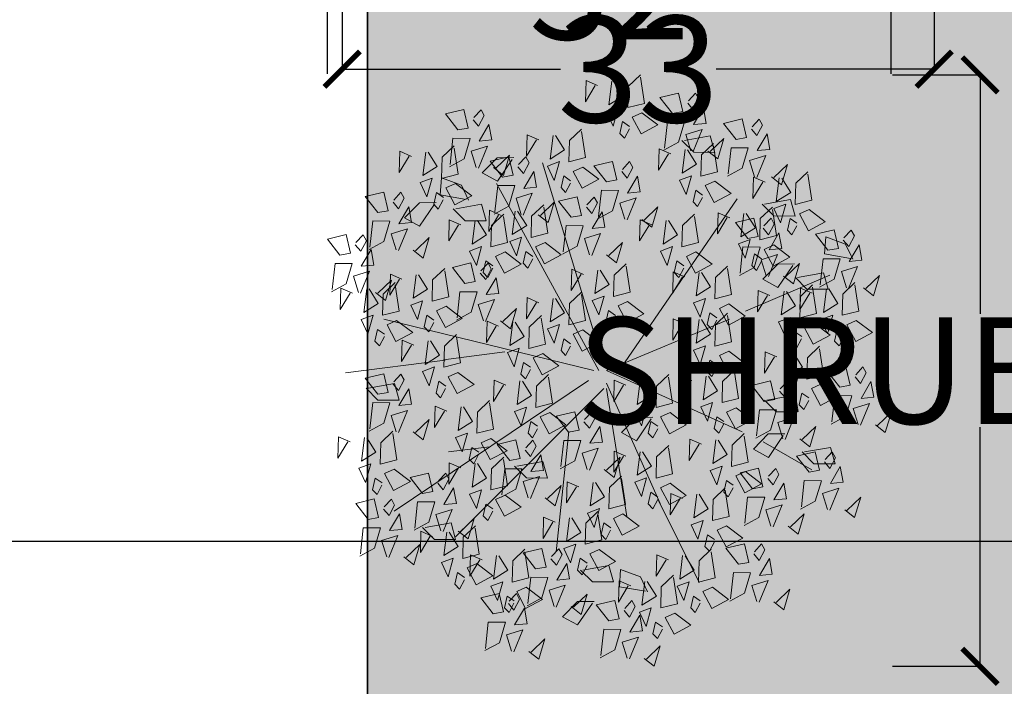
# Model space of a CAD drawing. Units: inches. Extents: x 1704 to 6393, y -157 to 1172.
# Tile 10 of 122: x 1879 to 1934, y 82 to 120. Entities that reach past the tile are written whole.
import ezdxf

# ---------------------------------------------------------------- set-up
doc = ezdxf.new("R2010")
doc.units = ezdxf.units.IN
doc.header["$MEASUREMENT"] = 0
for name, color, linetype, lineweight in [('A-ANNO-DIMS', 7, 'Continuous', 13), ('C-PROP', 7, 'Continuous', 35), ('L-shrub', 74, 'Continuous', 18)]:
    doc.layers.add(name, color=color, linetype=linetype, lineweight=lineweight)
doc.layers.add('L-PLNT-PATT', color=253, linetype='Continuous', lineweight=13, true_color=0x9abc8f)
doc.styles.get("Standard").update_dxf_attribs({"font": 'arial.ttf'})
doc.dimstyles.get("Standard").update_dxf_attribs({"dimtxt": 6, "dimasz": 2, "dimexe": 0.18, "dimexo": 0.0625, "dimgap": 0.09, "dimtad": 0, "dimtih": 1, "dimtoh": 1, "dimdec": 1, "dimzin": 0, "dimdsep": 46, "dimlunit": 3, "dimtxsty": 'Standard', "dimblk": 'ARCHTICK', "dimcen": 0.09, "dimadec": 0, "dimazin": 0, "dimtfac": 1, "dimtdec": 1, "dimtofl": 0, "dimtmove": 0, "dimatfit": 3, "dimfxl": 1, "dimtolj": 1, "dimtzin": 0, "dimarcsym": 0})

# ---------------------------------------------------------------- blocks, each defined once
blk = doc.blocks.new('flower shrub 2')
at = {"layer": 'L-shrub'}
for p, q in [((-106.23, 211.82), (-92.99, 218)), ((-93.69, 216.06), (-97.6, 193.26)), ((-112.6, 194.32), (-106.23, 211.82)), ((71.95, 198.59), (86.43, 202.67)), ((75.99, 175.82), (71.95, 198.59)), ((86.43, 202.67), (86.36, 184.05)), ((-97.6, 193.26), (-112.6, 194.32)), ((-81.12, 192.39), (-66.64, 196.47)), ((-77.07, 169.62), (-81.12, 192.39)), ((-66.64, 196.47), (-66.71, 177.85)), ((86.36, 184.05), (75.99, 173.75)), ((-66.71, 177.85), (-77.08, 167.55)), ((-145.24, 163.47), (-130.76, 167.54)), ((-130.76, 167.54), (-130.83, 148.93)), ((-88.72, 152.29), (-88.87, 166.9)), ((-87.4, 165.46), (-68.26, 152.47)), ((26.45, 165.53), (40.92, 169.61)), ((30.49, 142.76), (26.45, 165.53)), ((40.92, 169.61), (40.85, 150.99)), ((-141.2, 140.7), (-145.24, 163.47)), ((60.21, 144.02), (60.06, 158.64)), ((61.53, 157.19), (80.67, 144.21)), ((-130.83, 148.93), (-141.21, 138.63)), ((-75.44, 139.25), (-88.72, 152.29)), ((-68.26, 152.47), (-75.44, 139.25)), ((40.85, 150.99), (30.48, 140.69)), ((73.5, 130.99), (60.21, 144.02)), ((80.67, 144.21), (73.5, 130.99)), ((-201.09, 93.22), (-186.61, 97.3)), ((-186.61, 97.3), (-186.68, 78.69)), ((-197.05, 70.45), (-201.09, 93.22)), ((-186.68, 78.69), (-197.06, 68.38)), ((45.73, 28.33), (45.58, 42.95)), ((47.06, 41.5), (66.19, 28.51)), ((185.43, 32.08), (198.67, 38.26)), ((197.96, 36.32), (194.06, 13.53)), ((59.02, 15.29), (45.73, 28.33)), ((66.19, 28.51), (59.02, 15.29)), ((179.06, 14.59), (185.43, 32.08)), ((194.06, 13.53), (179.06, 14.59)), ((175.38, 4.39), (189.86, 8.47)), ((179.42, -18.38), (175.38, 4.39)), ((189.86, 8.47), (189.78, -10.15)), ((189.78, -10.15), (179.41, -20.45)), ((207.07, -23.32), (206.92, -8.7)), ((208.4, -10.15), (227.53, -23.13)), ((220.36, -36.35), (207.07, -23.32)), ((227.53, -23.13), (220.36, -36.35)), ((84.36, -53.46), (98.84, -49.38)), ((98.84, -49.38), (98.77, -68)), ((88.41, -76.23), (84.36, -53.46)), ((98.77, -68), (88.4, -78.3)), ((-181.81, -93.56), (-181.96, -78.94)), ((-180.48, -80.39), (-161.34, -93.38)), ((-168.52, -106.6), (-181.81, -93.56)), ((-161.34, -93.38), (-168.52, -106.6)), ((-141.1, -107.17), (-126.62, -103.09)), ((-126.62, -103.09), (-126.7, -121.71)), ((-137.06, -129.94), (-141.1, -107.17)), ((-157.94, -124.93), (-144.7, -118.75)), ((-145.41, -120.69), (-149.31, -143.48)), ((-164.31, -142.42), (-157.94, -124.93)), ((-126.7, -121.71), (-137.07, -132.01)), ((138.15, -134.03), (152.62, -129.95)), ((142.19, -156.8), (138.15, -134.03)), ((152.62, -129.95), (152.55, -148.57)), ((-149.31, -143.48), (-164.31, -142.42)), ((-142.51, -161.74), (-142.65, -147.12)), ((-141.18, -148.57), (-122.04, -161.55)), ((152.55, -148.57), (142.18, -158.87)), ((-129.22, -174.77), (-142.51, -161.74)), ((-122.04, -161.55), (-129.22, -174.77)), ((16.1, -183.61), (30.58, -179.53)), ((30.58, -179.53), (30.51, -198.15)), ((20.14, -206.38), (16.1, -183.61)), ((30.51, -198.15), (20.14, -208.45))]:
    blk.add_line(p, q, dxfattribs=at)
for points in [[(52.15, 237.83), (59.05, 246.56), (41.2, 251.84), (52.74, 239.81)], [(-67.82, 227.5), (-60.92, 236.23), (-78.77, 241.51), (-67.23, 229.48)], [(-39.32, 221.12), (-28.59, 235.29), (-20.71, 220.61), (-35.41, 212.74), (-39.32, 221.12)], [(29.03, 225.28), (27.99, 236.36), (14.33, 233.94), (29.03, 225.28)], [(-90.95, 214.95), (-91.98, 226.03), (-105.64, 223.61), (-90.95, 214.95)], [(10.23, 220.07), (15.95, 224.84), (6.62, 229.76), (1.48, 226.97), (8.24, 220.66)], [(52.02, 222.79), (37.77, 218.39), (33.35, 232.62), (52.6, 224.77)], [(126.62, 210.97), (133.52, 219.7), (115.67, 224.99), (127.2, 212.95)], [(-109.75, 209.74), (-104.02, 214.51), (-113.35, 219.43), (-118.49, 216.64), (-111.73, 210.33)], [(-67.96, 212.46), (-82.2, 208.06), (-86.62, 222.29), (-67.37, 214.44)], [(-70.39, 219.89), (-47.54, 223.41), (-43.79, 208.84), (-62.4, 209.34), (-72.46, 219.95)], [(19.2, 206.65), (5.18, 195.71), (1.34, 211.93), (17.57, 215.74), (19.2, 206.65)], [(49.53, 199.82), (26.54, 202.32), (26.68, 217.36), (44.53, 212.08), (51.52, 199.24)], [(-27.19, 210.46), (-31.5, 204.37), (-21.21, 202.03), (-16.97, 206.05), (-25.13, 210.4)], [(103.49, 198.43), (102.46, 209.5), (88.8, 207.08), (103.49, 198.43)], [(-100.78, 196.32), (-114.8, 185.38), (-118.63, 201.6), (-102.4, 205.41), (-100.78, 196.32)], [(-70.44, 189.49), (-93.43, 191.99), (-93.29, 207.03), (-75.44, 201.75), (-68.45, 188.91)], [(-66.87, 197.06), (-54.24, 204.99), (-46.3, 192.37), (-66.93, 195)], [(-44.01, 200.58), (-40.16, 190.14), (-27.58, 196), (-44.01, 200.58)], [(16.53, 190.13), (27.26, 204.31), (35.14, 189.63), (20.44, 181.76), (16.53, 190.13)], [(84.69, 193.22), (90.42, 197.99), (81.09, 202.9), (75.95, 200.11), (82.71, 193.8)], [(126.48, 195.93), (112.24, 191.53), (107.82, 205.76), (127.07, 197.91)], [(-136.54, 179.8), (-125.81, 193.98), (-117.93, 179.3), (-132.63, 171.43), (-136.54, 179.8)], [(-47.57, 123.92), (-79, 197.93)], [(-37.25, 183.93), (-26.52, 198.11), (-18.64, 183.43), (-33.34, 175.56), (-37.25, 183.93)], [(-14.54, 188.9), (8.31, 192.42), (12.06, 177.85), (-6.55, 178.35), (-16.61, 188.96)], [(124, 172.97), (101.01, 175.46), (101.15, 190.5), (119, 185.22), (125.98, 172.38)], [(-167.61, 178.57), (-144.76, 182.09), (-141.01, 167.52), (-159.62, 168.02), (-169.68, 178.63)], [(-68.32, 182.7), (-45.47, 186.22), (-41.72, 171.65), (-60.33, 172.15), (-70.39, 182.76)], [(-63.13, 182.49), (-67.54, 172.28), (-48.93, 171.78), (-63.18, 180.43)], [(64.56, 171.72), (71.46, 180.45), (53.61, 185.73), (65.15, 173.7)], [(66.94, 139.62), (91.63, 182.23)], [(93.66, 179.79), (79.64, 168.86), (75.81, 185.07), (92.04, 188.89), (93.66, 179.79)], [(-25.12, 173.27), (-29.43, 167.19), (-19.14, 164.84), (-14.9, 168.86), (-23.06, 173.21)], [(-11.02, 166.07), (1.61, 174), (9.54, 161.38), (-11.08, 164.01)], [(28.66, 179.47), (24.35, 173.38), (34.64, 171.04), (38.88, 175.06), (30.72, 179.41)], [(141.1, 161.39), (148, 170.12), (130.14, 175.4), (141.68, 163.37)], [(-124.41, 169.14), (-128.72, 163.05), (-118.43, 160.71), (-114.19, 164.73), (-122.34, 169.08)], [(-78.16, 157.26), (-71.26, 165.99), (-89.12, 171.27), (-77.58, 159.24)], [(-64.8, 159.87), (-52.17, 167.8), (-44.24, 155.19), (-64.86, 157.81)], [(11.84, 169.59), (15.69, 159.15), (28.27, 165.01), (11.84, 169.59)], [(41.44, 159.17), (40.4, 170.25), (26.74, 167.83), (41.44, 159.17)], [(64.43, 156.68), (50.18, 152.28), (45.76, 166.51), (65.01, 158.66)], [(-165.04, 146.93), (-158.14, 155.66), (-175.99, 160.94), (-164.45, 148.91)], [(-164.09, 155.74), (-151.46, 163.67), (-143.52, 151.05), (-164.15, 153.68)], [(-141.23, 159.26), (-137.38, 148.82), (-124.8, 154.68), (-141.23, 159.26)], [(-101.29, 144.71), (-102.33, 155.79), (-115.98, 153.37), (-101.29, 144.71)], [(-105.51, 148.81), (-94.78, 162.99), (-86.9, 148.31), (-101.6, 140.44), (-105.51, 148.81)], [(-41.95, 163.39), (-38.09, 152.95), (-25.52, 158.81), (-41.95, 163.39)], [(22.64, 153.96), (28.36, 158.73), (19.03, 163.65), (13.89, 160.86), (20.65, 154.55)], [(117.97, 148.84), (116.93, 159.92), (103.28, 157.5), (117.97, 148.84)], [(140.96, 146.35), (126.72, 141.95), (122.3, 156.18), (141.55, 148.33)], [(207.29, 148.99), (214.19, 157.72), (196.34, 163.01), (207.88, 150.97)], [(-136.58, 147.58), (-113.73, 151.1), (-109.98, 136.53), (-128.59, 137.03), (-138.65, 147.64)], [(-120.09, 139.5), (-114.36, 144.27), (-123.69, 149.19), (-128.83, 146.4), (-122.07, 140.09)], [(-78.3, 142.22), (-92.54, 137.81), (-96.96, 152.05), (-77.71, 144.2)], [(-7.28, 151.5), (-11.69, 141.29), (6.92, 140.79), (-7.33, 149.44)], [(31.61, 140.54), (17.59, 129.6), (13.76, 145.82), (29.99, 149.63), (31.61, 140.54)], [(61.95, 133.71), (38.95, 136.21), (39.09, 151.25), (56.94, 145.97), (63.93, 133.13)], [(99.17, 143.63), (104.9, 148.4), (95.57, 153.32), (90.43, 150.53), (97.19, 144.22)], [(184.16, 136.45), (183.13, 147.53), (169.47, 145.1), (184.16, 136.45)], [(-206.97, 129.17), (-201.24, 133.94), (-210.57, 138.86), (-215.71, 136.07), (-208.95, 129.76)], [(-188.17, 134.38), (-189.2, 145.46), (-202.86, 143.04), (-188.17, 134.38)], [(-165.18, 131.89), (-179.42, 127.48), (-183.84, 141.72), (-164.59, 133.87)], [(-160.34, 141.17), (-164.76, 130.96), (-146.15, 130.46), (-160.4, 139.11)], [(-93.39, 138.15), (-97.69, 132.06), (-87.4, 129.72), (-83.16, 133.74), (-91.32, 138.09)], [(-61.06, 145.31), (-65.47, 135.09), (-46.86, 134.59), (-61.11, 143.24)], [(108.14, 130.21), (94.12, 119.27), (90.29, 135.49), (106.52, 139.3), (108.14, 130.21)], [(93.06, 124.02), (103.79, 138.2), (111.67, 123.52), (96.98, 115.65), (93.06, 124.02)], [(138.48, 123.38), (115.49, 125.88), (115.63, 140.92), (133.48, 135.64), (140.46, 122.8)], [(165.36, 131.24), (171.09, 136.01), (161.76, 140.92), (156.62, 138.13), (163.38, 131.82)], [(207.15, 133.95), (192.91, 129.55), (188.49, 143.78), (207.74, 135.93)], [(-133.06, 124.75), (-120.43, 132.68), (-112.5, 120.06), (-133.12, 122.69)], [(-111.12, 126.07), (-125.14, 115.14), (-128.97, 131.36), (-112.74, 135.17), (-111.12, 126.07)], [(-80.78, 119.25), (-103.77, 121.75), (-103.63, 136.79), (-85.78, 131.5), (-78.8, 118.66)], [(37.21, 115.75), (47.94, 129.93), (55.82, 115.25), (41.13, 107.38), (37.21, 115.75)], [(-198, 115.75), (-212.02, 104.81), (-215.85, 121.03), (-199.62, 124.84), (-198, 115.75)], [(-167.66, 108.92), (-190.65, 111.42), (-190.51, 126.46), (-172.66, 121.17), (-165.67, 108.33)], [(-110.21, 128.27), (-106.35, 117.83), (-93.78, 123.69), (-110.21, 128.27)], [(-53.8, 109.56), (-43.07, 123.73), (-35.19, 109.05), (-49.89, 101.18), (-53.8, 109.56)], [(-12.43, 109.56), (-1.7, 123.73), (6.18, 109.05), (-8.52, 101.18), (-12.43, 109.56)], [(4.49, 2.24), (58.38, 121.09)], [(61.99, 122.79), (84.85, 126.31), (88.59, 111.74), (69.98, 112.24), (59.92, 122.85)], [(140.64, 107.49), (151.37, 121.67), (159.25, 106.99), (144.55, 99.12), (140.64, 107.49)], [(174.33, 117.81), (160.31, 106.88), (156.48, 123.09), (172.71, 126.91), (174.33, 117.81)], [(204.67, 110.99), (181.68, 113.48), (181.82, 128.52), (199.67, 123.24), (206.65, 110.4)], [(-2.25, 17.94), (-145.94, 116.61)], [(6.14, 114.53), (29, 118.04), (32.74, 103.47), (14.13, 103.98), (4.07, 114.58)], [(105.19, 113.36), (100.89, 107.27), (111.17, 104.93), (115.42, 108.95), (107.26, 113.3)], [(-187.79, 91.15), (-180.89, 99.88), (-198.75, 105.16), (-187.21, 93.13)], [(-161.36, 97.16), (-150.63, 111.34), (-142.75, 96.66), (-157.45, 88.79), (-161.36, 97.16)], [(-129.32, 110.18), (-133.73, 99.97), (-115.12, 99.47), (-129.37, 108.12)], [(-84.87, 108.33), (-62.02, 111.85), (-58.27, 97.28), (-76.88, 97.78), (-86.94, 108.38)], [(-43.5, 108.33), (-20.65, 111.85), (-16.9, 97.28), (-35.51, 97.78), (-45.57, 108.38)], [(4.49, 2.24), (-40.41, 109.88)], [(49.34, 105.09), (45.04, 99.01), (55.32, 96.67), (59.57, 100.68), (51.41, 105.04)], [(65.51, 99.96), (78.14, 107.89), (86.08, 95.27), (65.46, 97.9)], [(109.57, 106.26), (132.42, 109.78), (136.17, 95.21), (117.56, 95.71), (107.5, 106.32)], [(194.42, 95.09), (205.15, 109.27), (213.03, 94.59), (198.33, 86.72), (194.42, 95.09)], [(-192.43, 95.93), (-169.58, 99.45), (-165.83, 84.88), (-184.44, 85.38), (-194.5, 95.99)], [(-41.67, 98.9), (-45.98, 92.81), (-35.69, 90.47), (-31.45, 94.49), (-39.6, 98.84)], [(-0.3, 98.9), (-4.61, 92.81), (5.68, 90.47), (9.92, 94.49), (1.76, 98.84)], [(9.66, 91.7), (22.29, 99.62), (30.23, 87.01), (9.61, 89.63)], [(32.52, 95.21), (36.38, 84.78), (48.95, 90.64), (32.52, 95.21)], [(88.37, 103.48), (92.23, 93.04), (104.8, 98.9), (88.37, 103.48)], [(152.77, 96.83), (148.46, 90.75), (158.75, 88.4), (162.99, 92.42), (154.83, 96.77)], [(163.35, 93.87), (186.2, 97.38), (189.95, 82.82), (171.34, 83.32), (161.28, 93.92)], [(-210.92, 78.6), (-211.96, 89.68), (-225.62, 87.26), (-210.92, 78.6)], [(-149.23, 86.5), (-153.54, 80.42), (-143.25, 78.07), (-139.01, 82.09), (-147.17, 86.44)], [(-99.31, 80.63), (-88.58, 94.81), (-80.7, 80.13), (-95.39, 72.26), (-99.31, 80.63)], [(-81.35, 85.5), (-68.72, 93.43), (-60.78, 80.81), (-81.41, 83.43)], [(-58.49, 89.02), (-54.64, 78.58), (-42.06, 84.44), (-58.49, 89.02)], [(-39.98, 85.5), (-27.35, 93.43), (-19.41, 80.81), (-40.04, 83.43)], [(-17.12, 89.02), (-13.27, 78.58), (-0.69, 84.44), (-17.12, 89.02)], [(113.09, 83.43), (125.72, 91.36), (133.65, 78.75), (113.03, 81.37)], [(135.94, 86.95), (139.8, 76.51), (152.38, 82.37), (135.94, 86.95)], [(-229.72, 73.39), (-223.99, 78.16), (-233.32, 83.08), (-238.46, 80.29), (-231.7, 73.98)], [(-187.93, 76.11), (-202.17, 71.7), (-206.59, 85.94), (-187.34, 78.09)], [(-188.91, 73.1), (-176.28, 81.03), (-168.35, 68.42), (-188.97, 71.04)], [(-130.38, 79.41), (-107.52, 82.92), (-103.78, 68.35), (-122.39, 68.86), (-132.45, 79.46)], [(69.26, 85.39), (64.84, 75.18), (83.45, 74.68), (69.2, 83.33)], [(118.58, 47.68), (190.43, 83.56)], [(166.87, 71.04), (179.5, 78.96), (187.44, 66.35), (166.81, 68.97)], [(206.55, 84.43), (202.24, 78.35), (212.53, 76.01), (216.77, 80.02), (208.61, 84.38)], [(-220.75, 59.96), (-234.77, 49.03), (-238.6, 65.25), (-222.37, 69.06), (-220.75, 59.96)], [(-190.41, 53.14), (-213.4, 55.64), (-213.26, 70.68), (-195.41, 65.39), (-188.43, 52.55)], [(-166.05, 76.62), (-162.2, 66.18), (-149.62, 72.04), (-166.05, 76.62)], [(-87.18, 69.97), (-91.48, 63.89), (-81.2, 61.54), (-76.95, 65.56), (-85.11, 69.92)], [(-77.6, 70.93), (-82.02, 60.72), (-63.41, 60.22), (-77.66, 68.87)], [(-36.23, 70.93), (-40.65, 60.72), (-22.04, 60.22), (-36.29, 68.87)], [(13.41, 77.13), (8.99, 66.92), (27.6, 66.41), (13.35, 75.06)], [(41.35, 57.91), (52.08, 72.09), (59.96, 57.41), (45.26, 49.54), (41.35, 57.91)], [(103.41, 57.91), (114.13, 72.09), (122.01, 57.41), (107.32, 49.54), (103.41, 57.91)], [(189.73, 74.55), (193.58, 64.12), (206.16, 69.98), (189.73, 74.55)], [(217.17, 62.04), (227.9, 76.22), (235.78, 61.54), (221.08, 53.67), (217.17, 62.04)], [(-126.86, 56.58), (-114.23, 64.5), (-106.29, 51.89), (-126.91, 54.51)], [(116.83, 68.87), (112.42, 58.65), (131.03, 58.15), (116.78, 66.8)], [(186.1, 60.81), (208.96, 64.33), (212.7, 49.76), (194.09, 50.26), (184.03, 60.87)], [(-185.17, 58.54), (-189.58, 48.32), (-170.97, 47.82), (-185.22, 56.47)], [(-104, 60.09), (-100.14, 49.66), (-87.57, 55.52), (-104, 60.09)], [(10.28, 56.68), (33.14, 60.2), (36.88, 45.63), (18.27, 46.13), (8.21, 56.74)], [(72.33, 56.68), (95.19, 60.2), (98.94, 45.63), (80.33, 46.13), (70.27, 56.74)], [(170.61, 56.47), (166.2, 46.26), (184.81, 45.75), (170.56, 54.41)], [(-221.35, 33.12), (-210.62, 47.29), (-202.74, 32.61), (-217.44, 24.74), (-221.35, 33.12)], [(-127.81, 33.3), (-120.91, 42.03), (-138.76, 47.31), (-127.22, 35.28)], [(15.72, 2.24), (121.24, 49.33)], [(53.48, 47.25), (49.18, 41.16), (59.46, 38.82), (63.71, 42.84), (55.55, 47.19)], [(115.53, 47.25), (111.23, 41.16), (121.51, 38.82), (125.76, 42.84), (117.6, 47.19)], [(189.62, 37.98), (202.25, 45.91), (210.19, 33.29), (189.57, 35.92)], [(229.3, 51.38), (225, 45.3), (235.28, 42.95), (239.53, 46.97), (231.37, 51.32)], [(256.93, 35.37), (263.83, 44.1), (245.98, 49.38), (257.52, 37.35)], [(-252.42, 31.89), (-229.56, 35.41), (-225.82, 20.84), (-244.43, 21.34), (-254.49, 31.94)], [(-123.11, 42.01), (-127.53, 31.79), (-108.92, 31.29), (-123.17, 39.94)], [(-55.87, 20.72), (-45.14, 34.9), (-37.26, 20.22), (-51.96, 12.35), (-55.87, 20.72)], [(13.8, 33.85), (26.43, 41.78), (34.37, 29.16), (13.74, 31.79)], [(36.66, 37.37), (40.51, 26.93), (53.09, 32.79), (36.66, 37.37)], [(75.86, 33.85), (88.48, 41.78), (96.42, 29.16), (75.8, 31.79)], [(98.71, 37.37), (102.57, 26.93), (115.14, 32.79), (98.71, 37.37)], [(212.48, 41.5), (216.34, 31.06), (228.91, 36.92), (212.48, 41.5)], [(-150.93, 20.75), (-151.97, 31.83), (-165.63, 29.41), (-150.93, 20.75)], [(-127.94, 18.26), (-142.19, 13.86), (-146.61, 28.09), (-127.36, 20.24)], [(130.3, 16.59), (141.02, 30.77), (148.91, 16.09), (134.21, 8.22), (130.3, 16.59)], [(215.01, 17.61), (220.73, 22.38), (211.4, 27.3), (206.26, 24.51), (213.02, 18.2)], [(233.81, 22.82), (232.77, 33.9), (219.11, 31.48), (233.81, 22.82)], [(256.8, 20.33), (242.55, 15.92), (238.13, 30.16), (257.38, 22.31)], [(-209.22, 22.46), (-213.52, 16.37), (-203.24, 14.03), (-198.99, 18.05), (-207.15, 22.4)], [(-169.73, 15.55), (-164.01, 20.31), (-173.34, 25.23), (-178.48, 22.44), (-171.72, 16.13)], [(-86.94, 19.49), (-64.08, 23.01), (-60.34, 8.44), (-78.95, 8.94), (-89.01, 19.55)], [(17.55, 19.28), (13.13, 9.07), (31.74, 8.57), (17.49, 17.22)], [(20.21, 2.24), (132.47, 20.18)], [(79.6, 19.28), (75.19, 9.07), (93.8, 8.57), (79.54, 17.22)], [(99.22, 15.36), (122.08, 18.88), (125.83, 4.31), (107.22, 4.81), (97.16, 15.42)], [(193.37, 23.42), (188.95, 13.2), (207.56, 12.7), (193.31, 21.35)], [(-248.9, 9.06), (-236.27, 16.99), (-228.33, 4.37), (-248.95, 7)], [(-226.04, 12.58), (-222.18, 2.14), (-209.61, 8), (-226.04, 12.58)], [(-160.76, 2.12), (-174.78, -8.81), (-178.61, 7.4), (-162.38, 11.22), (-160.76, 2.12)], [(-130.42, -4.7), (-153.42, -2.21), (-153.28, 12.83), (-135.43, 7.55), (-128.44, -5.29)], [(-96.78, 2.31), (-89.88, 11.04), (-107.73, 16.33), (-96.19, 4.29)], [(-43.74, 10.06), (-48.04, 3.98), (-37.76, 1.63), (-33.51, 5.65), (-41.67, 10)], [(91.45, 0.25), (98.35, 8.98), (80.5, 14.26), (92.04, 2.23)], [(161.32, -4.07), (172.05, 10.11), (179.93, -4.57), (165.24, -12.44), (161.32, -4.07)], [(223.98, 4.18), (209.96, -6.75), (206.13, 9.47), (222.35, 13.28), (223.98, 4.18)], [(254.32, -2.64), (231.32, -0.14), (231.46, 14.9), (249.31, 9.61), (256.3, -3.23)], [(0, 0), (-177.37, -53.82)], [(-119.91, -10.23), (-120.94, 0.84), (-134.6, -1.58), (-119.91, -10.23)], [(-83.42, -3.34), (-70.79, 4.59), (-62.85, -8.02), (-83.47, -5.4)], [(-60.56, 0.18), (-56.71, -10.26), (-44.13, -4.4), (-60.56, 0.18)], [(20.21, 0), (150.43, -130.06)], [(102.75, -7.47), (115.38, 0.46), (123.31, -12.16), (102.69, -9.53)], [(142.42, 5.93), (138.12, -0.16), (148.4, -2.5), (152.65, 1.52), (144.49, 5.87)], [(-245.15, -5.51), (-249.57, -15.72), (-230.96, -16.22), (-245.21, -7.57)], [(-173.77, -18.53), (-163.04, -4.35), (-155.16, -19.03), (-169.86, -26.9), (-173.77, -18.53)], [(4.49, -4.48), (-159.41, -94.18)], [(-138.71, -15.44), (-132.98, -10.67), (-142.31, -5.76), (-147.45, -8.55), (-140.69, -14.86)], [(-96.92, -12.73), (-111.16, -17.13), (-115.58, -2.9), (-96.33, -10.75)], [(-31.05, -18.53), (-20.32, -4.35), (-12.44, -19.03), (-27.13, -26.9), (-31.05, -18.53)], [(49.53, -17.51), (55.25, -12.74), (45.92, -7.82), (40.78, -10.61), (47.54, -16.92)], [(68.33, -12.3), (67.29, -1.22), (53.63, -3.64), (68.33, -12.3)], [(91.32, -14.79), (77.07, -19.2), (72.66, -4.96), (91.9, -12.81)], [(125.6, -3.95), (129.46, -14.39), (142.03, -8.53), (125.6, -3.95)], [(130.25, -5.3), (153.11, -1.78), (156.85, -16.35), (138.24, -15.85), (128.18, -5.24)], [(-204.84, -19.76), (-181.99, -16.24), (-178.24, -30.81), (-196.85, -30.31), (-206.91, -19.7)], [(-62.12, -19.76), (-39.26, -16.24), (-35.52, -30.81), (-54.13, -30.31), (-64.19, -19.7)], [(4.49, -8.97), (-40.41, -192.85)], [(13.47, -13.45), (127.98, -183.88)], [(173.45, -14.73), (169.15, -20.81), (179.43, -23.16), (183.68, -19.14), (175.52, -14.79)], [(211.43, -28.68), (218.32, -19.95), (200.47, -14.66), (212.01, -26.7)], [(-129.74, -28.87), (-143.76, -39.8), (-147.59, -23.59), (-131.36, -19.77), (-129.74, -28.87)], [(-99.4, -35.69), (-122.39, -33.2), (-122.25, -18.16), (-104.4, -23.44), (-97.41, -36.28)], [(-79.67, -17.9), (-84.09, -28.12), (-65.48, -28.62), (-79.73, -19.97)], [(58.5, -30.94), (44.48, -41.87), (40.65, -25.65), (56.88, -21.84), (58.5, -30.94)], [(88.84, -37.76), (65.84, -35.27), (65.98, -20.22), (83.83, -25.51), (90.82, -38.35)], [(106.49, -22.04), (102.08, -32.25), (120.69, -32.75), (106.44, -24.1)], [(133.77, -28.13), (146.4, -20.2), (154.34, -32.82), (133.72, -30.19)], [(156.63, -24.61), (160.49, -35.05), (173.06, -29.19), (156.63, -24.61)], [(-161.65, -29.19), (-165.95, -35.28), (-155.67, -37.62), (-151.42, -33.6), (-159.58, -29.25)], [(-18.92, -29.19), (-23.22, -35.28), (-12.94, -37.62), (-8.69, -33.6), (-16.85, -29.25)], [(41.35, -47.45), (52.08, -33.28), (59.96, -47.96), (45.26, -55.83), (41.35, -47.45)], [(57.96, -30.81), (163.48, -42.02)], [(188.3, -41.22), (187.26, -30.14), (173.6, -32.57), (188.3, -41.22)], [(211.29, -43.72), (197.04, -48.12), (192.63, -33.89), (211.88, -41.74)], [(-201.32, -42.59), (-188.69, -34.66), (-180.76, -47.28), (-201.38, -44.65)], [(-178.47, -39.07), (-174.61, -49.51), (-162.04, -43.65), (-178.47, -39.07)], [(-107.58, -51.59), (-96.85, -37.41), (-88.97, -52.09), (-103.67, -59.96), (-107.58, -51.59)], [(-58.6, -42.59), (-45.97, -34.66), (-38.03, -47.28), (-58.65, -44.65)], [(-35.74, -39.07), (-31.88, -49.51), (-19.31, -43.65), (-35.74, -39.07)], [(-10.36, -53.65), (0.37, -39.48), (8.25, -54.15), (-6.45, -62.02), (-10.36, -53.65)], [(116.28, -51.4), (123.17, -42.67), (105.32, -37.39), (116.86, -49.42)], [(137.52, -42.69), (133.1, -52.91), (151.71, -53.41), (137.46, -44.76)], [(169.5, -46.43), (175.23, -41.66), (165.89, -36.75), (160.76, -39.54), (167.52, -45.85)], [(-131.94, -57.6), (-125.04, -48.87), (-142.9, -43.59), (-131.36, -55.62)], [(-138.65, -52.81), (-115.8, -49.3), (-112.05, -63.87), (-130.66, -63.36), (-140.72, -52.76)], [(-41.43, -54.88), (-18.58, -51.36), (-14.83, -65.93), (-33.44, -65.43), (-43.5, -54.82)], [(10.28, -48.68), (33.14, -45.17), (36.88, -59.73), (18.27, -59.23), (8.21, -48.63)], [(178.47, -59.86), (164.45, -70.79), (160.62, -54.58), (176.85, -50.76), (178.47, -59.86)], [(208.81, -66.68), (185.82, -64.19), (185.95, -49.15), (203.81, -54.43), (210.79, -67.27)], [(-197.58, -57.16), (-201.99, -67.37), (-183.38, -67.87), (-197.63, -59.22)], [(-155.07, -70.15), (-156.11, -59.07), (-169.77, -61.49), (-155.07, -70.15)], [(-54.85, -57.16), (-59.27, -67.37), (-40.66, -67.87), (-54.91, -59.22)], [(53.48, -58.12), (49.18, -64.2), (59.46, -66.54), (63.71, -62.52), (55.55, -58.17)], [(74.35, -69.16), (80.08, -64.39), (70.74, -59.47), (65.6, -62.26), (72.37, -68.57)], [(93.15, -63.95), (92.11, -52.87), (78.45, -55.29), (93.15, -63.95)], [(116.14, -66.44), (101.89, -70.85), (97.48, -56.61), (116.73, -64.46)], [(194.42, -68.11), (205.15, -53.94), (213.03, -68.62), (198.33, -76.49), (194.42, -68.11)], [(250.73, -65.86), (257.63, -57.13), (239.78, -51.85), (251.31, -63.88)], [(-173.87, -75.36), (-168.14, -70.59), (-177.47, -65.67), (-182.61, -68.46), (-175.85, -74.77)], [(-132.08, -72.64), (-146.33, -77.04), (-150.74, -62.81), (-131.49, -70.66)], [(-135.13, -75.64), (-122.5, -67.72), (-114.56, -80.33), (-135.19, -77.71)], [(-95.45, -62.25), (-99.76, -68.33), (-89.47, -70.68), (-85.23, -66.66), (-93.39, -62.3)], [(1.77, -64.31), (-2.54, -70.4), (7.75, -72.74), (11.99, -68.72), (3.83, -64.37)], [(13.8, -71.51), (26.43, -63.59), (34.37, -76.2), (13.74, -73.58)], [(36.66, -67.99), (40.51, -78.43), (53.09, -72.57), (36.66, -67.99)], [(163.35, -69.34), (186.2, -65.83), (189.95, -80.39), (171.34, -79.89), (161.28, -69.29)], [(227.6, -78.41), (226.56, -67.33), (212.91, -69.75), (227.6, -78.41)], [(-112.27, -72.13), (-108.42, -82.56), (-95.84, -76.7), (-112.27, -72.13)], [(-99.31, -86.71), (-88.58, -72.53), (-80.7, -87.21), (-95.39, -95.08), (-99.31, -86.71)], [(-38.86, -90.66), (-31.96, -81.92), (-49.81, -76.64), (-38.27, -88.67)], [(-37.91, -77.71), (-25.28, -69.78), (-17.35, -82.4), (-37.97, -79.77)], [(-15.06, -74.19), (-11.2, -84.63), (1.38, -78.77), (-15.06, -74.19)], [(83.32, -82.58), (69.3, -93.52), (65.47, -77.3), (81.7, -73.49), (83.32, -82.58)], [(113.66, -89.41), (90.67, -86.91), (90.8, -71.87), (108.65, -77.16), (115.64, -90)], [(113.75, -86.71), (124.48, -72.53), (132.36, -87.21), (117.66, -95.08), (113.75, -86.71)], [(208.8, -83.62), (214.53, -78.85), (205.2, -73.93), (200.06, -76.72), (206.82, -83.03)], [(250.59, -80.9), (236.35, -85.31), (231.93, -71.07), (251.18, -78.92)], [(-173.31, -96.85), (-166.41, -88.12), (-184.27, -82.84), (-172.73, -94.87)], [(-164.9, -88.78), (-178.92, -99.72), (-182.75, -83.5), (-166.52, -79.68), (-164.9, -88.78)], [(-134.56, -95.61), (-157.55, -93.11), (-157.42, -78.07), (-139.56, -83.35), (-132.58, -96.19)], [(-130.38, -87.94), (-107.52, -84.42), (-103.78, -98.99), (-122.39, -98.48), (-132.45, -87.88)], [(17.55, -86.08), (13.13, -96.29), (31.74, -96.8), (17.49, -88.14)], [(64.1, -99.1), (74.83, -84.93), (82.71, -99.61), (68.02, -107.48), (64.1, -99.1)], [(82.68, -87.94), (105.53, -84.42), (109.28, -98.99), (90.67, -98.48), (80.61, -87.88)], [(166.87, -92.17), (179.5, -84.24), (187.44, -96.86), (166.81, -94.24)], [(206.55, -78.77), (202.24, -84.86), (212.53, -87.2), (216.77, -83.18), (208.61, -78.83)], [(-131.39, -90.21), (-135.8, -100.43), (-117.19, -100.93), (-131.44, -92.28)], [(-61.99, -103.2), (-63.02, -92.12), (-76.68, -94.54), (-61.99, -103.2)], [(-34.17, -92.28), (-38.58, -102.49), (-19.97, -102.99), (-34.22, -94.34)], [(-4.91, -140.69), (-11.65, -86.87)], [(189.73, -88.65), (193.58, -99.09), (206.16, -93.23), (189.73, -88.65)], [(217.77, -97.05), (203.75, -107.98), (199.92, -91.76), (216.15, -87.95), (217.77, -97.05)], [(248.11, -103.87), (225.12, -101.38), (225.26, -86.33), (243.11, -91.62), (250.09, -104.46)], [(-196.44, -109.4), (-197.48, -98.32), (-211.14, -100.74), (-196.44, -109.4)], [(-173.45, -111.89), (-187.7, -116.3), (-192.11, -102.06), (-172.86, -109.91)], [(-126.86, -110.76), (-114.23, -102.84), (-106.29, -115.45), (-126.91, -112.83)], [(-87.18, -97.37), (-91.48, -103.45), (-81.2, -105.8), (-76.95, -101.78), (-85.11, -97.42)], [(-80.79, -108.41), (-75.06, -103.64), (-84.39, -98.73), (-89.53, -101.51), (-82.77, -107.82)], [(-39, -105.7), (-53.24, -110.1), (-57.66, -95.86), (-38.41, -103.72)], [(33.03, -100.33), (55.89, -96.81), (59.63, -111.38), (41.02, -110.88), (30.96, -100.28)], [(71.43, -100.32), (75.92, -136.2)], [(86.2, -110.76), (98.83, -102.84), (106.76, -115.45), (86.14, -112.83)], [(125.88, -97.37), (121.57, -103.45), (131.86, -105.8), (136.1, -101.78), (127.94, -97.42)], [(173.73, -111.5), (184.46, -97.32), (192.34, -112), (177.65, -119.87), (173.73, -111.5)], [(-215.24, -114.61), (-209.51, -109.84), (-218.84, -104.92), (-223.98, -107.71), (-217.22, -114.02)], [(-104, -107.25), (-100.14, -117.69), (-87.57, -111.82), (-104, -107.25)], [(-41.48, -128.66), (-64.47, -126.17), (-64.33, -111.13), (-46.48, -116.41), (-39.5, -129.25)], [(76.23, -109.76), (71.93, -115.85), (82.21, -118.19), (86.46, -114.17), (78.3, -109.82)], [(109.05, -107.25), (112.91, -117.69), (125.48, -111.82), (109.05, -107.25)], [(142.66, -112.73), (165.52, -109.21), (169.26, -123.78), (150.65, -123.28), (140.59, -112.67)], [(170.61, -106.74), (166.2, -116.95), (184.81, -117.46), (170.56, -108.8)], [(-206.27, -128.04), (-220.29, -138.97), (-224.12, -122.75), (-207.89, -118.94), (-206.27, -128.04)], [(-175.93, -134.86), (-198.92, -132.36), (-198.79, -117.32), (-180.93, -122.61), (-173.95, -135.45)], [(-159.29, -130.09), (-148.56, -115.91), (-140.68, -130.59), (-155.38, -138.46), (-159.29, -130.09)], [(-71.82, -121.84), (-85.84, -132.77), (-89.67, -116.56), (-73.44, -112.74), (-71.82, -121.84)], [(6.19, -128.03), (16.91, -113.85), (24.8, -128.53), (10.1, -136.4), (6.19, -128.03)], [(36.55, -123.16), (49.18, -115.23), (57.12, -127.85), (36.5, -125.22)], [(59.41, -119.64), (63.27, -130.08), (75.84, -124.22), (59.41, -119.64)], [(145.23, -127.84), (152.13, -119.11), (134.28, -113.83), (145.82, -125.86)], [(-190.37, -131.32), (-167.51, -127.8), (-163.76, -142.37), (-182.37, -141.87), (-192.43, -131.26)], [(-123.11, -125.33), (-127.53, -135.55), (-108.92, -136.05), (-123.17, -127.4)], [(-51.73, -138.36), (-41, -124.18), (-33.12, -138.86), (-47.82, -146.73), (-51.73, -138.36)], [(-24.89, -129.25), (-2.03, -125.74), (1.72, -140.31), (-16.89, -139.8), (-26.95, -129.2)], [(89.94, -125.33), (85.53, -135.55), (104.14, -136.05), (89.89, -127.4)], [(122.11, -140.39), (121.07, -129.31), (107.41, -131.73), (122.11, -140.39)], [(146.18, -135.56), (158.81, -127.63), (166.75, -140.24), (146.13, -137.62)], [(185.86, -122.16), (181.56, -128.24), (191.84, -130.59), (196.09, -126.57), (187.93, -122.22)], [(-82.8, -139.58), (-59.95, -136.07), (-56.2, -150.64), (-74.81, -150.13), (-84.87, -139.53)], [(40.3, -137.73), (35.89, -147.94), (54.49, -148.44), (40.24, -139.79)], [(103.31, -145.6), (109.03, -140.83), (99.7, -135.91), (94.56, -138.7), (101.33, -145.01)], [(145.1, -142.88), (130.85, -147.29), (126.44, -133.05), (145.68, -140.9)], [(169.04, -132.04), (172.9, -142.48), (185.47, -136.62), (169.04, -132.04)], [(-186.84, -154.15), (-174.21, -146.22), (-166.28, -158.84), (-186.9, -156.21)], [(-147.17, -140.75), (-151.47, -146.84), (-141.19, -149.18), (-136.94, -145.16), (-145.1, -140.81)], [(-21.36, -152.08), (-8.73, -144.16), (-0.8, -156.77), (-21.42, -154.15)], [(-4.49, -139.03), (6.74, -226.49)], [(18.31, -138.69), (14.01, -144.77), (24.29, -147.12), (28.54, -143.1), (20.38, -138.74)], [(-163.99, -150.63), (-160.13, -161.07), (-147.56, -155.21), (-163.99, -150.63)], [(-100.92, -167.09), (-94.02, -158.36), (-111.87, -153.08), (-100.33, -165.11)], [(-79.28, -162.41), (-66.65, -154.49), (-58.72, -167.1), (-79.34, -164.48)], [(-39.6, -149.02), (-43.91, -155.1), (-33.62, -157.44), (-29.38, -153.43), (-37.54, -149.07)], [(1.49, -148.57), (5.35, -159), (17.92, -153.14), (1.49, -148.57)], [(58.36, -167.09), (65.26, -158.36), (47.41, -153.08), (58.94, -165.11)], [(112.28, -159.02), (98.26, -169.96), (94.43, -153.74), (110.66, -149.93), (112.28, -159.02)], [(142.62, -165.85), (119.63, -163.35), (119.76, -148.31), (137.61, -153.6), (144.6, -166.44)], [(149.93, -150.12), (145.52, -160.34), (164.12, -160.84), (149.87, -152.19)], [(-56.42, -158.9), (-52.57, -169.33), (-39.99, -163.47), (-56.42, -158.9)], [(167.99, -175.36), (174.89, -166.63), (157.04, -161.34), (168.57, -173.38)], [(-183.1, -168.72), (-187.51, -178.93), (-168.9, -179.43), (-183.15, -170.78)], [(-124.04, -179.64), (-125.08, -168.56), (-138.74, -170.98), (-124.04, -179.64)], [(-101.05, -182.14), (-115.3, -186.54), (-119.71, -172.3), (-100.47, -180.15)], [(-39.32, -181.74), (-28.59, -167.56), (-20.71, -182.24), (-35.41, -190.11), (-39.32, -181.74)], [(-17.62, -166.65), (-22.03, -176.87), (-3.42, -177.37), (-17.67, -168.72)], [(35.23, -179.64), (34.2, -168.56), (20.54, -170.98), (35.23, -179.64)], [(58.22, -182.14), (43.98, -186.54), (39.56, -172.3), (58.81, -180.15)], [(90.99, -183.81), (101.72, -169.63), (109.6, -184.31), (94.91, -192.18), (90.99, -183.81)], [(-142.84, -184.85), (-137.12, -180.08), (-146.45, -175.17), (-151.59, -177.95), (-144.83, -184.26)], [(-75.54, -176.98), (-79.95, -187.19), (-61.34, -187.7), (-75.59, -179.05)], [(-70.39, -182.97), (-47.54, -179.45), (-43.79, -194.02), (-62.4, -193.52), (-72.46, -182.91)], [(16.43, -184.85), (22.16, -180.08), (12.83, -175.17), (7.69, -177.95), (14.45, -184.26)], [(144.86, -187.9), (143.83, -176.83), (130.17, -179.25), (144.86, -187.9)], [(167.85, -190.4), (153.61, -194.8), (149.19, -180.57), (168.44, -188.42)], [(-133.87, -198.28), (-147.89, -209.21), (-151.72, -192.99), (-135.49, -189.18), (-133.87, -198.28)], [(-103.53, -205.1), (-126.52, -202.61), (-126.39, -187.57), (-108.54, -192.85), (-101.55, -205.69)], [(-63.68, -200.15), (-56.78, -191.42), (-74.64, -186.14), (-63.1, -198.17)], [(25.4, -198.28), (11.38, -209.21), (7.55, -192.99), (23.78, -189.18), (25.4, -198.28)], [(55.74, -205.1), (32.75, -202.61), (32.89, -187.57), (50.74, -192.85), (57.72, -205.69)], [(59.92, -185.03), (82.78, -181.52), (86.52, -196.09), (67.91, -195.58), (57.85, -184.98)], [(126.06, -193.11), (131.79, -188.35), (122.46, -183.43), (117.32, -186.22), (124.08, -192.53)], [(-66.87, -205.8), (-54.24, -197.87), (-46.3, -210.49), (-66.93, -207.86)], [(-27.19, -192.4), (-31.5, -198.49), (-21.21, -200.83), (-16.97, -196.81), (-25.13, -192.46)], [(103.12, -194.47), (98.82, -200.55), (109.1, -202.9), (113.35, -198.88), (105.19, -194.52)], [(135.03, -206.54), (121.01, -217.47), (117.18, -201.26), (133.41, -197.44), (135.03, -206.54)], [(165.37, -213.36), (142.38, -210.87), (142.52, -195.83), (160.37, -201.11), (167.35, -213.95)], [(-86.81, -212.7), (-87.85, -201.62), (-101.51, -204.04), (-86.81, -212.7)], [(-63.82, -215.19), (-78.07, -219.59), (-82.48, -205.36), (-63.23, -213.21)], [(-44.01, -202.28), (-40.16, -212.72), (-27.58, -206.86), (-44.01, -202.28)], [(63.44, -207.86), (76.07, -199.94), (84.01, -212.55), (63.39, -209.93)], [(86.3, -204.35), (90.16, -214.78), (102.73, -208.92), (86.3, -204.35)], [(-105.61, -217.91), (-99.88, -213.14), (-109.21, -208.22), (-114.35, -211.01), (-107.59, -217.32)], [(-96.64, -231.33), (-110.66, -242.26), (-114.49, -226.05), (-98.26, -222.23), (-96.64, -231.33)], [(-66.3, -238.16), (-89.29, -235.66), (-89.16, -220.62), (-71.3, -225.9), (-64.32, -238.74)], [(-63.13, -220.37), (-67.54, -230.58), (-48.93, -231.08), (-63.18, -222.43)], [(67.19, -222.43), (62.78, -232.65), (81.39, -233.15), (67.13, -224.5)]]:
    blk.add_lwpolyline(points, dxfattribs=at)
blk = doc.blocks.new('_ArchTick')
at = {"color": 0, "linetype": 'ByBlock', "const_width": 0.15}
blk.add_lwpolyline([(-0.5, -0.5), (0.5, 0.5)], dxfattribs=at)
blk = doc.blocks.new('*D79')
at = {"layer": 'A-ANNO-DIMS', "color": 0, "lineweight": -2, "transparency": 16777216}
for p, q in [((1896.932, 121.786), (1896.932, 116.659)), ((1930.289, 121.786), (1930.289, 116.659)), ((1896.932, 116.839), (1909.225, 116.839)), ((1930.289, 116.839), (1917.996, 116.839))]:
    blk.add_line(p, q, dxfattribs=at)
at = {"layer": 'Defpoints', "color": 0, "lineweight": -3, "transparency": 16777216}
for p in [(1896.932, 121.849), (1930.289, 121.849), (1930.289, 116.839)]:
    blk.add_point(p, dxfattribs=at)
at = {"layer": 'A-ANNO-DIMS', "color": 0, "lineweight": -2, "transparency": 16777216, "xscale": 2, "yscale": 2, "zscale": 2, "rotation": 180}
blk.add_blockref('_ArchTick', (1896.932, 116.839), dxfattribs=at)
at = {"layer": 'A-ANNO-DIMS', "color": 0, "lineweight": -2, "transparency": 16777216, "xscale": 2, "yscale": 2, "zscale": 2}
blk.add_blockref('_ArchTick', (1930.289, 116.839), dxfattribs=at)
at = {"layer": 'A-ANNO-DIMS', "color": 0, "transparency": 16777216, "insert": (1913.611, 116.839), "char_height": 6, "attachment_point": 5}
blk.add_mtext('\\A1;33', dxfattribs=at)
blk = doc.blocks.new('*D82')
at = {"layer": 'A-ANNO-DIMS', "color": 0, "lineweight": -2, "transparency": 16777216}
for p, q in [((1927.934, 116.512), (1933.05, 116.512)), ((1932.87, 116.512), (1932.87, 103.044)), ((1932.87, 83.187), (1932.87, 96.655)), ((1927.934, 83.187), (1933.05, 83.187))]:
    blk.add_line(p, q, dxfattribs=at)
at = {"layer": 'Defpoints', "color": 0, "lineweight": -3, "transparency": 16777216}
for p in [(1927.871, 116.512), (1927.871, 83.187), (1932.87, 83.187)]:
    blk.add_point(p, dxfattribs=at)
at = {"layer": 'A-ANNO-DIMS', "color": 0, "lineweight": -2, "transparency": 16777216, "xscale": 2, "yscale": 2, "zscale": 2}
for p, rotation in [((1932.87, 116.512), 90), ((1932.87, 83.187), 270)]:
    blk.add_blockref('_ArchTick', p, dxfattribs=dict(at, rotation=rotation))
at = {"layer": 'A-ANNO-DIMS', "color": 0, "transparency": 16777216, "insert": (1932.87, 99.849), "char_height": 6, "attachment_point": 5}
blk.add_mtext('\\A1;SHRUB B 33', dxfattribs=at)
blk = doc.blocks.new('*D83')
at = {"layer": 'A-ANNO-DIMS', "color": 0, "lineweight": -2, "transparency": 16777216}
for p, q in [((1896.102, 116.575), (1896.102, 121.691)), ((1896.102, 121.511), (1907.632, 121.511)), ((1927.871, 121.511), (1916.342, 121.511)), ((1927.871, 116.575), (1927.871, 121.691))]:
    blk.add_line(p, q, dxfattribs=at)
at = {"layer": 'Defpoints', "color": 0, "lineweight": -3, "transparency": 16777216}
for p in [(1927.871, 121.511), (1896.102, 116.512), (1927.871, 116.512)]:
    blk.add_point(p, dxfattribs=at)
at = {"layer": 'A-ANNO-DIMS', "color": 0, "lineweight": -2, "transparency": 16777216, "xscale": 2, "yscale": 2, "zscale": 2, "rotation": 180}
blk.add_blockref('_ArchTick', (1896.102, 121.511), dxfattribs=at)
at = {"layer": 'A-ANNO-DIMS', "color": 0, "lineweight": -2, "transparency": 16777216, "xscale": 2, "yscale": 2, "zscale": 2}
blk.add_blockref('_ArchTick', (1927.871, 121.511), dxfattribs=at)
at = {"layer": 'A-ANNO-DIMS', "color": 0, "transparency": 16777216, "insert": (1911.987, 121.511), "char_height": 6, "attachment_point": 5}
blk.add_mtext('\\A1;32', dxfattribs=at)
blk = doc.blocks.new('*D93')
at = {"layer": 'A-ANNO-DIMS', "color": 0, "lineweight": -2, "transparency": 16777216}
for p, q in [((2605.286, 895.213), (1829.698, 895.213)), ((1829.878, 895.213), (1829.878, 495.866)), ((1829.878, 90.213), (1829.878, 489.56)), ((2605.286, 90.213), (1829.698, 90.213))]:
    blk.add_line(p, q, dxfattribs=at)
at = {"layer": 'Defpoints', "color": 0, "lineweight": -3, "transparency": 16777216}
for p in [(2605.349, 895.213), (1829.878, 90.213), (2605.349, 90.213)]:
    blk.add_point(p, dxfattribs=at)
at = {"layer": 'A-ANNO-DIMS', "color": 0, "lineweight": -2, "transparency": 16777216, "xscale": 2, "yscale": 2, "zscale": 2}
for p, rotation in [((1829.878, 895.213), 90), ((1829.878, 90.213), 270)]:
    blk.add_blockref('_ArchTick', p, dxfattribs=dict(at, rotation=rotation))
at = {"layer": 'A-ANNO-DIMS', "color": 0, "transparency": 16777216, "insert": (1829.878, 492.713), "char_height": 6, "attachment_point": 5}
blk.add_mtext('\\A1;805', dxfattribs=at)

msp = doc.modelspace()

# ---------------------------------------------------------------- hatches: boundary and pattern name
at = {"layer": 'L-PLNT-PATT', "transparency": 33554643}
h = msp.add_hatch(color=256, dxfattribs=at)
h.dxf.hatch_style = 1
h.paths.add_polyline_path([(1975.349, 202.213), (1898.349, 202.213), (1898.349, -3.787), (1975.349, -3.787)])

# ---------------------------------------------------------------- linework, layer by layer
at = {"layer": 'C-PROP'}
msp.add_line((1898.349, -3.787), (1898.349, 1033.213), dxfattribs=at)

# ---------------------------------------------------------------- block references
at = {"layer": 'L-shrub', "xscale": 0.0642956299502212, "yscale": 0.0642956299502212, "zscale": 0.0642956299502212, "rotation": 270}
msp.add_blockref('flower shrub 2', (1911.679, 100.15), dxfattribs=at)

# ---------------------------------------------------------------- dimensions: what is measured, and where the dimension line sits
at = {"layer": 'A-ANNO-DIMS'}
dim = msp.add_linear_dim(base=(1829.878, 90.213), p1=(2605.349, 895.213), p2=(2605.349, 90.213), angle=90, dimstyle='Standard', override={"dimdec": 0, "dimlfac": 1, "dimrnd": 0, "dimzin": 0, "dimdsep": 46, "dimlunit": 2}, dxfattribs=at)
dim.commit()
dim.dimension.update_dxf_attribs({"geometry": '*D93', "text_midpoint": (1829.878, 492.713)})
for base, p1, p2, picture, middle in [((1927.871, 121.511), (1896.102, 116.512), (1927.871, 116.512), '*D83', (1911.987, 121.511)), ((1930.289, 116.839), (1896.932, 121.849), (1930.289, 121.849), '*D79', (1913.611, 116.839))]:
    dim = msp.add_linear_dim(base=base, p1=p1, p2=p2, dimstyle='Standard', override={"dimdec": 0, "dimlfac": 1, "dimrnd": 0, "dimzin": 0, "dimdsep": 46, "dimlunit": 2}, dxfattribs=at)
    dim.commit()
    dim.dimension.update_dxf_attribs({"geometry": picture, "text_midpoint": middle})
dim = msp.add_linear_dim(base=(1932.87, 83.187), p1=(1927.871, 116.512), p2=(1927.871, 83.187), angle=270, text='SHRUB B <>', dimstyle='Standard', override={"dimdec": 0, "dimlfac": 1, "dimrnd": 0, "dimzin": 0, "dimdsep": 46, "dimlunit": 2}, dxfattribs=at)
dim.commit()
dim.dimension.update_dxf_attribs({"geometry": '*D82', "text_midpoint": (1932.87, 99.849)})

doc.saveas('drawing.dxf')
